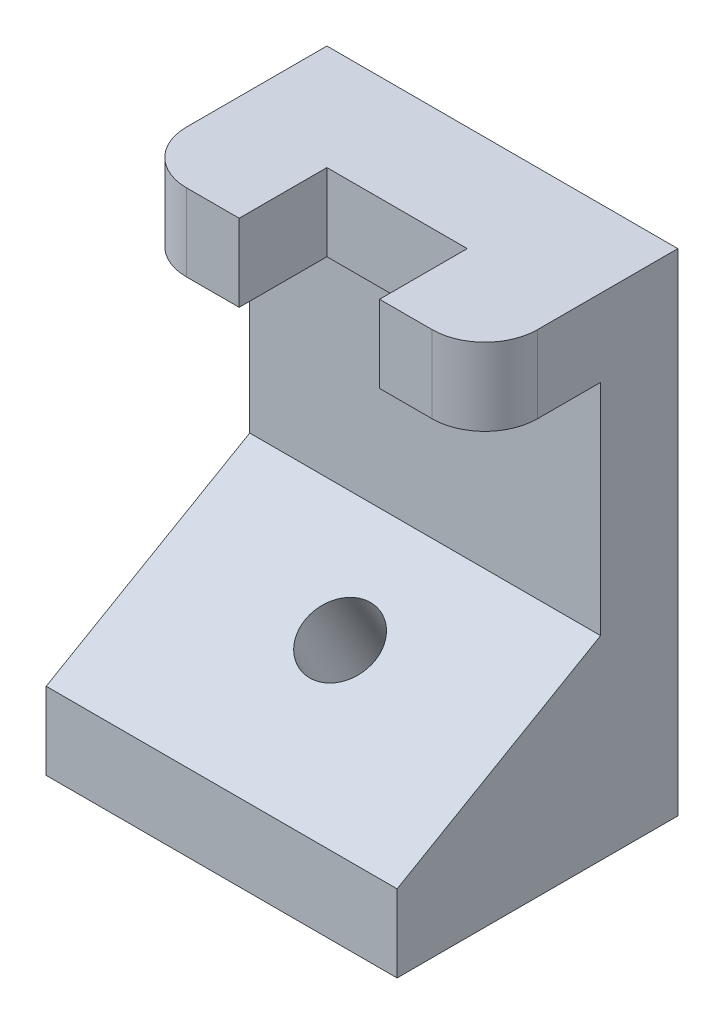
ISO-10303-21;
HEADER;
FILE_DESCRIPTION(('STEP AP214'),'2;1');
FILE_NAME('part.step','',(''),(''),'','','');
FILE_SCHEMA(('AUTOMOTIVE_DESIGN { 1 0 10303 214 1 1 1 1 }'));
ENDSEC;
DATA;
#1=APPLICATION_CONTEXT('core data for automotive mechanical design processes');
#2=APPLICATION_PROTOCOL_DEFINITION('international standard','automotive_design',2000,#1);
#3=PRODUCT_CONTEXT('',#1,'mechanical');
#4=PRODUCT('Part','Part','',(#3));
#5=PRODUCT_RELATED_PRODUCT_CATEGORY('part','',(#4));
#6=PRODUCT_DEFINITION_FORMATION('','',#4);
#7=PRODUCT_DEFINITION_CONTEXT('part definition',#1,'design');
#8=PRODUCT_DEFINITION('design','',#6,#7);
#9=PRODUCT_DEFINITION_SHAPE('','',#8);
#10=(LENGTH_UNIT() NAMED_UNIT(*) SI_UNIT(.MILLI.,.METRE.));
#11=(NAMED_UNIT(*) PLANE_ANGLE_UNIT() SI_UNIT($,.RADIAN.));
#12=(NAMED_UNIT(*) SI_UNIT($,.STERADIAN.) SOLID_ANGLE_UNIT());
#13=UNCERTAINTY_MEASURE_WITH_UNIT(LENGTH_MEASURE(1.E-05),#10,'distance_accuracy_value','');
#14=(GEOMETRIC_REPRESENTATION_CONTEXT(3) GLOBAL_UNCERTAINTY_ASSIGNED_CONTEXT((#13)) GLOBAL_UNIT_ASSIGNED_CONTEXT((#10,
#11,#12)) REPRESENTATION_CONTEXT('',''));
#15=CARTESIAN_POINT('',(0.,0.,0.));
#16=DIRECTION('',(0.,0.,1.));
#17=DIRECTION('',(1.,0.,0.));
#18=AXIS2_PLACEMENT_3D('',#15,#16,#17);
#19=CARTESIAN_POINT('',(1.,2.8,-0.500000000000001));
#20=DIRECTION('',(0.,0.,-1.));
#21=DIRECTION('',(-1.,0.,0.));
#22=AXIS2_PLACEMENT_3D('',#19,#20,#21);
#23=PLANE('',#22);
#24=DIRECTION('',(-1.,0.,0.));
#25=VECTOR('',#24,1.);
#26=CARTESIAN_POINT('',(1.,2.36,-0.500000000000001));
#27=LINE('',#26,#25);
#28=CARTESIAN_POINT('',(0.7,2.36,-0.500000000000001));
#29=VERTEX_POINT('',#28);
#30=CARTESIAN_POINT('',(0.4,2.36,-0.500000000000001));
#31=VERTEX_POINT('',#30);
#32=EDGE_CURVE('E222',#29,#31,#27,.T.);
#33=ORIENTED_EDGE('',*,*,#32,.F.);
#34=DIRECTION('',(0.,-1.,0.));
#35=VECTOR('',#34,1.);
#36=CARTESIAN_POINT('',(0.7,2.8,-0.500000000000001));
#37=LINE('',#36,#35);
#38=CARTESIAN_POINT('',(0.7,2.8,-0.500000000000001));
#39=VERTEX_POINT('',#38);
#40=EDGE_CURVE('E246',#29,#39,#37,.F.);
#41=ORIENTED_EDGE('',*,*,#40,.T.);
#42=DIRECTION('',(-1.,0.,0.));
#43=VECTOR('',#42,1.);
#44=CARTESIAN_POINT('',(1.,2.8,-0.500000000000001));
#45=LINE('',#44,#43);
#46=CARTESIAN_POINT('',(0.4,2.8,-0.500000000000001));
#47=VERTEX_POINT('',#46);
#48=EDGE_CURVE('E221',#39,#47,#45,.T.);
#49=ORIENTED_EDGE('',*,*,#48,.T.);
#50=DIRECTION('',(0.,1.,0.));
#51=VECTOR('',#50,1.);
#52=CARTESIAN_POINT('',(0.4,1.8,-0.500000000000001));
#53=LINE('',#52,#51);
#54=EDGE_CURVE('E163',#31,#47,#53,.T.);
#55=ORIENTED_EDGE('',*,*,#54,.F.);
#56=EDGE_LOOP('',(#33,#41,#49,#55));
#57=FACE_BOUND('',#56,.T.);
#58=ADVANCED_FACE('F44',(#57),#23,.F.);
#59=CARTESIAN_POINT('',(1.,0.,0.));
#60=DIRECTION('',(0.,0.,-1.));
#61=DIRECTION('',(-1.,0.,0.));
#62=AXIS2_PLACEMENT_3D('',#59,#60,#61);
#63=PLANE('',#62);
#64=DIRECTION('',(0.,-1.,0.));
#65=VECTOR('',#64,1.);
#66=CARTESIAN_POINT('',(-1.,0.,0.));
#67=LINE('',#66,#65);
#68=CARTESIAN_POINT('',(-1.,0.44,0.));
#69=VERTEX_POINT('',#68);
#70=CARTESIAN_POINT('',(-1.,0.,0.));
#71=VERTEX_POINT('',#70);
#72=EDGE_CURVE('E176',#69,#71,#67,.T.);
#73=ORIENTED_EDGE('',*,*,#72,.T.);
#74=DIRECTION('',(-1.,0.,0.));
#75=VECTOR('',#74,1.);
#76=CARTESIAN_POINT('',(1.,0.,0.));
#77=LINE('',#76,#75);
#78=CARTESIAN_POINT('',(1.,0.,0.));
#79=VERTEX_POINT('',#78);
#80=EDGE_CURVE('E235',#79,#71,#77,.T.);
#81=ORIENTED_EDGE('',*,*,#80,.F.);
#82=DIRECTION('',(0.,-1.,0.));
#83=VECTOR('',#82,1.);
#84=CARTESIAN_POINT('',(1.,0.,0.));
#85=LINE('',#84,#83);
#86=CARTESIAN_POINT('',(1.,0.44,0.));
#87=VERTEX_POINT('',#86);
#88=EDGE_CURVE('E182',#87,#79,#85,.T.);
#89=ORIENTED_EDGE('',*,*,#88,.F.);
#90=DIRECTION('',(-1.,0.,0.));
#91=VECTOR('',#90,1.);
#92=CARTESIAN_POINT('',(1.,0.44,0.));
#93=LINE('',#92,#91);
#94=EDGE_CURVE('E196',#87,#69,#93,.T.);
#95=ORIENTED_EDGE('',*,*,#94,.T.);
#96=EDGE_LOOP('',(#73,#81,#89,#95));
#97=FACE_BOUND('',#96,.T.);
#98=ADVANCED_FACE('F274',(#97),#63,.F.);
#99=CARTESIAN_POINT('',(1.,0.,0.));
#100=DIRECTION('',(0.,1.,0.));
#101=DIRECTION('',(0.,0.,1.));
#102=AXIS2_PLACEMENT_3D('',#99,#100,#101);
#103=PLANE('',#102);
#104=CARTESIAN_POINT('',(0.,0.,-1.15406848361773));
#105=DIRECTION('',(0.,1.,0.));
#106=DIRECTION('',(0.,0.,1.));
#107=AXIS2_PLACEMENT_3D('',#104,#105,#106);
#108=ELLIPSE('',#107,0.230940107675851,0.2);
#109=CARTESIAN_POINT('',(0.,0.,-0.923128375941875));
#110=VERTEX_POINT('',#109);
#111=EDGE_CURVE('E170',#110,#110,#108,.T.);
#112=ORIENTED_EDGE('',*,*,#111,.T.);
#113=EDGE_LOOP('',(#112));
#114=FACE_BOUND('',#113,.T.);
#115=DIRECTION('',(0.,0.,-1.));
#116=VECTOR('',#115,1.);
#117=CARTESIAN_POINT('',(-1.,0.,0.));
#118=LINE('',#117,#116);
#119=CARTESIAN_POINT('',(-1.,0.,-1.6));
#120=VERTEX_POINT('',#119);
#121=EDGE_CURVE('E203',#71,#120,#118,.T.);
#122=ORIENTED_EDGE('',*,*,#121,.T.);
#123=DIRECTION('',(-1.,0.,0.));
#124=VECTOR('',#123,1.);
#125=CARTESIAN_POINT('',(1.,0.,-1.6));
#126=LINE('',#125,#124);
#127=CARTESIAN_POINT('',(1.,0.,-1.6));
#128=VERTEX_POINT('',#127);
#129=EDGE_CURVE('E226',#128,#120,#126,.T.);
#130=ORIENTED_EDGE('',*,*,#129,.F.);
#131=DIRECTION('',(0.,0.,-1.));
#132=VECTOR('',#131,1.);
#133=CARTESIAN_POINT('',(1.,0.,0.));
#134=LINE('',#133,#132);
#135=EDGE_CURVE('E184',#79,#128,#134,.T.);
#136=ORIENTED_EDGE('',*,*,#135,.F.);
#137=ORIENTED_EDGE('',*,*,#80,.T.);
#138=EDGE_LOOP('',(#122,#130,#136,#137));
#139=FACE_BOUND('',#138,.T.);
#140=ADVANCED_FACE('F282',(#114,#139),#103,.F.);
#141=CARTESIAN_POINT('',(1.,0.,-1.6));
#142=DIRECTION('',(0.,0.,1.));
#143=DIRECTION('',(1.,0.,0.));
#144=AXIS2_PLACEMENT_3D('',#141,#142,#143);
#145=PLANE('',#144);
#146=DIRECTION('',(0.,1.,0.));
#147=VECTOR('',#146,1.);
#148=CARTESIAN_POINT('',(-1.,0.,-1.6));
#149=LINE('',#148,#147);
#150=CARTESIAN_POINT('',(-1.,2.8,-1.6));
#151=VERTEX_POINT('',#150);
#152=EDGE_CURVE('E201',#120,#151,#149,.T.);
#153=ORIENTED_EDGE('',*,*,#152,.T.);
#154=DIRECTION('',(-1.,0.,0.));
#155=VECTOR('',#154,1.);
#156=CARTESIAN_POINT('',(1.,2.8,-1.6));
#157=LINE('',#156,#155);
#158=CARTESIAN_POINT('',(1.,2.8,-1.6));
#159=VERTEX_POINT('',#158);
#160=EDGE_CURVE('E227',#159,#151,#157,.T.);
#161=ORIENTED_EDGE('',*,*,#160,.F.);
#162=DIRECTION('',(0.,1.,0.));
#163=VECTOR('',#162,1.);
#164=CARTESIAN_POINT('',(1.,0.,-1.6));
#165=LINE('',#164,#163);
#166=EDGE_CURVE('E189',#128,#159,#165,.T.);
#167=ORIENTED_EDGE('',*,*,#166,.F.);
#168=ORIENTED_EDGE('',*,*,#129,.T.);
#169=EDGE_LOOP('',(#153,#161,#167,#168));
#170=FACE_BOUND('',#169,.T.);
#171=ADVANCED_FACE('F294',(#170),#145,.F.);
#172=CARTESIAN_POINT('',(1.,2.8,-1.6));
#173=DIRECTION('',(0.,-1.,0.));
#174=DIRECTION('',(0.,0.,-1.));
#175=AXIS2_PLACEMENT_3D('',#172,#173,#174);
#176=PLANE('',#175);
#177=DIRECTION('',(0.,0.,1.));
#178=VECTOR('',#177,1.);
#179=CARTESIAN_POINT('',(-1.,2.8,-1.6));
#180=LINE('',#179,#178);
#181=CARTESIAN_POINT('',(-1.,2.8,-0.800000000000001));
#182=VERTEX_POINT('',#181);
#183=EDGE_CURVE('E202',#151,#182,#180,.T.);
#184=ORIENTED_EDGE('',*,*,#183,.T.);
#185=CARTESIAN_POINT('',(-0.7,2.8,-0.800000000000001));
#186=DIRECTION('',(0.,-1.,0.));
#187=DIRECTION('',(0.,0.,-1.));
#188=AXIS2_PLACEMENT_3D('',#185,#186,#187);
#189=CIRCLE('',#188,0.3);
#190=CARTESIAN_POINT('',(-0.7,2.8,-0.500000000000001));
#191=VERTEX_POINT('',#190);
#192=EDGE_CURVE('E11',#182,#191,#189,.F.);
#193=ORIENTED_EDGE('',*,*,#192,.T.);
#194=CARTESIAN_POINT('',(-0.4,2.8,-0.500000000000001));
#195=VERTEX_POINT('',#194);
#196=EDGE_CURVE('E224',#195,#191,#45,.T.);
#197=ORIENTED_EDGE('',*,*,#196,.F.);
#198=DIRECTION('',(0.,0.,1.));
#199=VECTOR('',#198,1.);
#200=CARTESIAN_POINT('',(-0.4,2.8,-1.));
#201=LINE('',#200,#199);
#202=CARTESIAN_POINT('',(-0.4,2.8,-1.));
#203=VERTEX_POINT('',#202);
#204=EDGE_CURVE('E160',#203,#195,#201,.T.);
#205=ORIENTED_EDGE('',*,*,#204,.F.);
#206=DIRECTION('',(-1.,0.,0.));
#207=VECTOR('',#206,1.);
#208=CARTESIAN_POINT('',(0.4,2.8,-1.));
#209=LINE('',#208,#207);
#210=CARTESIAN_POINT('',(0.4,2.8,-1.));
#211=VERTEX_POINT('',#210);
#212=EDGE_CURVE('E149',#211,#203,#209,.T.);
#213=ORIENTED_EDGE('',*,*,#212,.F.);
#214=DIRECTION('',(0.,0.,-1.));
#215=VECTOR('',#214,1.);
#216=CARTESIAN_POINT('',(0.4,2.8,-1.));
#217=LINE('',#216,#215);
#218=EDGE_CURVE('E161',#47,#211,#217,.T.);
#219=ORIENTED_EDGE('',*,*,#218,.F.);
#220=ORIENTED_EDGE('',*,*,#48,.F.);
#221=CARTESIAN_POINT('',(0.7,2.8,-0.800000000000001));
#222=DIRECTION('',(0.,-1.,0.));
#223=DIRECTION('',(0.,0.,-1.));
#224=AXIS2_PLACEMENT_3D('',#221,#222,#223);
#225=CIRCLE('',#224,0.3);
#226=CARTESIAN_POINT('',(1.,2.8,-0.800000000000001));
#227=VERTEX_POINT('',#226);
#228=EDGE_CURVE('E247',#39,#227,#225,.F.);
#229=ORIENTED_EDGE('',*,*,#228,.T.);
#230=DIRECTION('',(0.,0.,1.));
#231=VECTOR('',#230,1.);
#232=CARTESIAN_POINT('',(1.,2.8,-1.6));
#233=LINE('',#232,#231);
#234=EDGE_CURVE('E186',#159,#227,#233,.T.);
#235=ORIENTED_EDGE('',*,*,#234,.F.);
#236=ORIENTED_EDGE('',*,*,#160,.T.);
#237=EDGE_LOOP('',(#184,#193,#197,#205,#213,#219,#220,#229,#235,#236));
#238=FACE_BOUND('',#237,.T.);
#239=ADVANCED_FACE('F166',(#238),#176,.F.);
#240=ORIENTED_EDGE('',*,*,#196,.T.);
#241=DIRECTION('',(0.,-1.,0.));
#242=VECTOR('',#241,1.);
#243=CARTESIAN_POINT('',(-0.7,2.36,-0.500000000000001));
#244=LINE('',#243,#242);
#245=CARTESIAN_POINT('',(-0.7,2.36,-0.500000000000001));
#246=VERTEX_POINT('',#245);
#247=EDGE_CURVE('E249',#191,#246,#244,.T.);
#248=ORIENTED_EDGE('',*,*,#247,.T.);
#249=CARTESIAN_POINT('',(-0.4,2.36,-0.500000000000001));
#250=VERTEX_POINT('',#249);
#251=EDGE_CURVE('E219',#250,#246,#27,.T.);
#252=ORIENTED_EDGE('',*,*,#251,.F.);
#253=DIRECTION('',(0.,1.,0.));
#254=VECTOR('',#253,1.);
#255=CARTESIAN_POINT('',(-0.4,1.8,-0.500000000000001));
#256=LINE('',#255,#254);
#257=EDGE_CURVE('E180',#250,#195,#256,.T.);
#258=ORIENTED_EDGE('',*,*,#257,.T.);
#259=EDGE_LOOP('',(#240,#248,#252,#258));
#260=FACE_BOUND('',#259,.T.);
#261=ADVANCED_FACE('F260',(#260),#23,.F.);
#262=CARTESIAN_POINT('',(1.,2.36,-0.500000000000001));
#263=DIRECTION('',(0.,1.,0.));
#264=DIRECTION('',(0.,0.,1.));
#265=AXIS2_PLACEMENT_3D('',#262,#263,#264);
#266=PLANE('',#265);
#267=ORIENTED_EDGE('',*,*,#251,.T.);
#268=CARTESIAN_POINT('',(-0.7,2.36,-0.800000000000001));
#269=DIRECTION('',(0.,1.,0.));
#270=DIRECTION('',(0.,0.,1.));
#271=AXIS2_PLACEMENT_3D('',#268,#269,#270);
#272=CIRCLE('',#271,0.3);
#273=CARTESIAN_POINT('',(-1.,2.36,-0.8));
#274=VERTEX_POINT('',#273);
#275=EDGE_CURVE('E70',#246,#274,#272,.F.);
#276=ORIENTED_EDGE('',*,*,#275,.T.);
#277=DIRECTION('',(0.,0.,-1.));
#278=VECTOR('',#277,1.);
#279=CARTESIAN_POINT('',(-1.,2.36,-0.500000000000001));
#280=LINE('',#279,#278);
#281=CARTESIAN_POINT('',(-1.,2.36,-1.16));
#282=VERTEX_POINT('',#281);
#283=EDGE_CURVE('E210',#274,#282,#280,.T.);
#284=ORIENTED_EDGE('',*,*,#283,.T.);
#285=DIRECTION('',(-1.,0.,0.));
#286=VECTOR('',#285,1.);
#287=CARTESIAN_POINT('',(1.,2.36,-1.16));
#288=LINE('',#287,#286);
#289=CARTESIAN_POINT('',(1.,2.36,-1.16));
#290=VERTEX_POINT('',#289);
#291=EDGE_CURVE('E220',#290,#282,#288,.T.);
#292=ORIENTED_EDGE('',*,*,#291,.F.);
#293=DIRECTION('',(0.,0.,-1.));
#294=VECTOR('',#293,1.);
#295=CARTESIAN_POINT('',(1.,2.36,-0.500000000000001));
#296=LINE('',#295,#294);
#297=CARTESIAN_POINT('',(1.,2.36,-0.8));
#298=VERTEX_POINT('',#297);
#299=EDGE_CURVE('E195',#298,#290,#296,.T.);
#300=ORIENTED_EDGE('',*,*,#299,.F.);
#301=CARTESIAN_POINT('',(0.7,2.36,-0.800000000000001));
#302=DIRECTION('',(0.,1.,0.));
#303=DIRECTION('',(0.,0.,1.));
#304=AXIS2_PLACEMENT_3D('',#301,#302,#303);
#305=CIRCLE('',#304,0.3);
#306=EDGE_CURVE('E241',#298,#29,#305,.F.);
#307=ORIENTED_EDGE('',*,*,#306,.T.);
#308=ORIENTED_EDGE('',*,*,#32,.T.);
#309=DIRECTION('',(0.,0.,-1.));
#310=VECTOR('',#309,1.);
#311=CARTESIAN_POINT('',(0.4,2.36,-0.500000000000001));
#312=LINE('',#311,#310);
#313=CARTESIAN_POINT('',(0.4,2.36,-1.));
#314=VERTEX_POINT('',#313);
#315=EDGE_CURVE('E239',#31,#314,#312,.T.);
#316=ORIENTED_EDGE('',*,*,#315,.T.);
#317=DIRECTION('',(-1.,0.,0.));
#318=VECTOR('',#317,1.);
#319=CARTESIAN_POINT('',(1.,2.36,-1.));
#320=LINE('',#319,#318);
#321=CARTESIAN_POINT('',(-0.4,2.36,-1.));
#322=VERTEX_POINT('',#321);
#323=EDGE_CURVE('E155',#314,#322,#320,.T.);
#324=ORIENTED_EDGE('',*,*,#323,.T.);
#325=DIRECTION('',(0.,0.,1.));
#326=VECTOR('',#325,1.);
#327=CARTESIAN_POINT('',(-0.4,2.36,-0.500000000000001));
#328=LINE('',#327,#326);
#329=EDGE_CURVE('E237',#322,#250,#328,.T.);
#330=ORIENTED_EDGE('',*,*,#329,.T.);
#331=EDGE_LOOP('',(#267,#276,#284,#292,#300,#307,#308,#316,#324,#330));
#332=FACE_BOUND('',#331,.T.);
#333=ADVANCED_FACE('F257',(#332),#266,.F.);
#334=CARTESIAN_POINT('',(1.,2.36,-1.16));
#335=DIRECTION('',(0.,0.,-1.));
#336=DIRECTION('',(0.,1.,0.));
#337=AXIS2_PLACEMENT_3D('',#334,#335,#336);
#338=PLANE('',#337);
#339=DIRECTION('',(0.,-1.,0.));
#340=VECTOR('',#339,1.);
#341=CARTESIAN_POINT('',(-1.,2.36,-1.16));
#342=LINE('',#341,#340);
#343=CARTESIAN_POINT('',(-1.,1.10972631225997,-1.16));
#344=VERTEX_POINT('',#343);
#345=EDGE_CURVE('E207',#282,#344,#342,.T.);
#346=ORIENTED_EDGE('',*,*,#345,.T.);
#347=DIRECTION('',(-1.,0.,0.));
#348=VECTOR('',#347,1.);
#349=CARTESIAN_POINT('',(1.,1.10972631225997,-1.16));
#350=LINE('',#349,#348);
#351=CARTESIAN_POINT('',(1.,1.10972631225997,-1.16));
#352=VERTEX_POINT('',#351);
#353=EDGE_CURVE('E212',#352,#344,#350,.T.);
#354=ORIENTED_EDGE('',*,*,#353,.F.);
#355=DIRECTION('',(0.,-1.,0.));
#356=VECTOR('',#355,1.);
#357=CARTESIAN_POINT('',(1.,2.36,-1.16));
#358=LINE('',#357,#356);
#359=EDGE_CURVE('E193',#290,#352,#358,.T.);
#360=ORIENTED_EDGE('',*,*,#359,.F.);
#361=ORIENTED_EDGE('',*,*,#291,.T.);
#362=EDGE_LOOP('',(#346,#354,#360,#361));
#363=FACE_BOUND('',#362,.T.);
#364=ADVANCED_FACE('F291',(#363),#338,.F.);
#365=CARTESIAN_POINT('',(1.,0.44,0.));
#366=DIRECTION('',(0.,-0.866025403784438,-0.500000000000001));
#367=DIRECTION('',(0.,0.500000000000001,-0.866025403784438));
#368=AXIS2_PLACEMENT_3D('',#365,#366,#367);
#369=PLANE('',#368);
#370=CARTESIAN_POINT('',(0.,0.829726312259968,-0.675025773880716));
#371=DIRECTION('',(0.,0.866025403784438,0.500000000000001));
#372=DIRECTION('',(0.,-0.500000000000001,0.866025403784438));
#373=AXIS2_PLACEMENT_3D('',#370,#371,#372);
#374=CIRCLE('',#373,0.2);
#375=CARTESIAN_POINT('',(0.,0.729726312259968,-0.501820693123828));
#376=VERTEX_POINT('',#375);
#377=EDGE_CURVE('E540',#376,#376,#374,.T.);
#378=ORIENTED_EDGE('',*,*,#377,.F.);
#379=EDGE_LOOP('',(#378));
#380=FACE_BOUND('',#379,.T.);
#381=DIRECTION('',(0.,-0.500000000000001,0.866025403784438));
#382=VECTOR('',#381,1.);
#383=CARTESIAN_POINT('',(-1.,0.44,0.));
#384=LINE('',#383,#382);
#385=EDGE_CURVE('E183',#344,#69,#384,.T.);
#386=ORIENTED_EDGE('',*,*,#385,.T.);
#387=ORIENTED_EDGE('',*,*,#94,.F.);
#388=DIRECTION('',(0.,-0.500000000000001,0.866025403784438));
#389=VECTOR('',#388,1.);
#390=CARTESIAN_POINT('',(1.,0.44,0.));
#391=LINE('',#390,#389);
#392=EDGE_CURVE('E198',#352,#87,#391,.T.);
#393=ORIENTED_EDGE('',*,*,#392,.F.);
#394=ORIENTED_EDGE('',*,*,#353,.T.);
#395=EDGE_LOOP('',(#386,#387,#393,#394));
#396=FACE_BOUND('',#395,.T.);
#397=ADVANCED_FACE('F322',(#380,#396),#369,.F.);
#398=CARTESIAN_POINT('',(1.,0.,0.));
#399=DIRECTION('',(-1.,0.,0.));
#400=DIRECTION('',(0.,0.,1.));
#401=AXIS2_PLACEMENT_3D('',#398,#399,#400);
#402=PLANE('',#401);
#403=ORIENTED_EDGE('',*,*,#234,.T.);
#404=DIRECTION('',(0.,-1.,0.));
#405=VECTOR('',#404,1.);
#406=CARTESIAN_POINT('',(1.,0.,-0.800000000000001));
#407=LINE('',#406,#405);
#408=EDGE_CURVE('E242',#227,#298,#407,.T.);
#409=ORIENTED_EDGE('',*,*,#408,.T.);
#410=ORIENTED_EDGE('',*,*,#299,.T.);
#411=ORIENTED_EDGE('',*,*,#359,.T.);
#412=ORIENTED_EDGE('',*,*,#392,.T.);
#413=ORIENTED_EDGE('',*,*,#88,.T.);
#414=ORIENTED_EDGE('',*,*,#135,.T.);
#415=ORIENTED_EDGE('',*,*,#166,.T.);
#416=EDGE_LOOP('',(#403,#409,#410,#411,#412,#413,#414,#415));
#417=FACE_BOUND('',#416,.T.);
#418=ADVANCED_FACE('F320',(#417),#402,.F.);
#419=CARTESIAN_POINT('',(-1.,0.,0.));
#420=DIRECTION('',(-1.,0.,0.));
#421=DIRECTION('',(0.,0.,1.));
#422=AXIS2_PLACEMENT_3D('',#419,#420,#421);
#423=PLANE('',#422);
#424=ORIENTED_EDGE('',*,*,#283,.F.);
#425=DIRECTION('',(0.,-1.,0.));
#426=VECTOR('',#425,1.);
#427=CARTESIAN_POINT('',(-1.,2.8,-0.800000000000001));
#428=LINE('',#427,#426);
#429=EDGE_CURVE('E52',#274,#182,#428,.F.);
#430=ORIENTED_EDGE('',*,*,#429,.T.);
#431=ORIENTED_EDGE('',*,*,#183,.F.);
#432=ORIENTED_EDGE('',*,*,#152,.F.);
#433=ORIENTED_EDGE('',*,*,#121,.F.);
#434=ORIENTED_EDGE('',*,*,#72,.F.);
#435=ORIENTED_EDGE('',*,*,#385,.F.);
#436=ORIENTED_EDGE('',*,*,#345,.F.);
#437=EDGE_LOOP('',(#424,#430,#431,#432,#433,#434,#435,#436));
#438=FACE_BOUND('',#437,.T.);
#439=ADVANCED_FACE('F314',(#438),#423,.T.);
#440=CARTESIAN_POINT('',(0.4,1.8,-1.));
#441=DIRECTION('',(1.,0.,0.));
#442=DIRECTION('',(0.,0.,-1.));
#443=AXIS2_PLACEMENT_3D('',#440,#441,#442);
#444=PLANE('',#443);
#445=ORIENTED_EDGE('',*,*,#54,.T.);
#446=ORIENTED_EDGE('',*,*,#218,.T.);
#447=DIRECTION('',(0.,1.,0.));
#448=VECTOR('',#447,1.);
#449=CARTESIAN_POINT('',(0.4,1.8,-1.));
#450=LINE('',#449,#448);
#451=EDGE_CURVE('E144',#314,#211,#450,.T.);
#452=ORIENTED_EDGE('',*,*,#451,.F.);
#453=ORIENTED_EDGE('',*,*,#315,.F.);
#454=EDGE_LOOP('',(#445,#446,#452,#453));
#455=FACE_BOUND('',#454,.T.);
#456=ADVANCED_FACE('F165',(#455),#444,.F.);
#457=CARTESIAN_POINT('',(-0.4,1.8,-1.));
#458=DIRECTION('',(-1.,0.,0.));
#459=DIRECTION('',(0.,0.,1.));
#460=AXIS2_PLACEMENT_3D('',#457,#458,#459);
#461=PLANE('',#460);
#462=DIRECTION('',(0.,1.,0.));
#463=VECTOR('',#462,1.);
#464=CARTESIAN_POINT('',(-0.4,1.8,-1.));
#465=LINE('',#464,#463);
#466=EDGE_CURVE('E156',#322,#203,#465,.T.);
#467=ORIENTED_EDGE('',*,*,#466,.T.);
#468=ORIENTED_EDGE('',*,*,#204,.T.);
#469=ORIENTED_EDGE('',*,*,#257,.F.);
#470=ORIENTED_EDGE('',*,*,#329,.F.);
#471=EDGE_LOOP('',(#467,#468,#469,#470));
#472=FACE_BOUND('',#471,.T.);
#473=ADVANCED_FACE('F263',(#472),#461,.F.);
#474=CARTESIAN_POINT('',(0.4,1.8,-1.));
#475=DIRECTION('',(0.,0.,-1.));
#476=DIRECTION('',(-1.,0.,0.));
#477=AXIS2_PLACEMENT_3D('',#474,#475,#476);
#478=PLANE('',#477);
#479=ORIENTED_EDGE('',*,*,#451,.T.);
#480=ORIENTED_EDGE('',*,*,#212,.T.);
#481=ORIENTED_EDGE('',*,*,#466,.F.);
#482=ORIENTED_EDGE('',*,*,#323,.F.);
#483=EDGE_LOOP('',(#479,#480,#481,#482));
#484=FACE_BOUND('',#483,.T.);
#485=ADVANCED_FACE('F150',(#484),#478,.F.);
#486=CARTESIAN_POINT('',(0.7,0.,-0.800000000000001));
#487=DIRECTION('',(0.,-1.,0.));
#488=DIRECTION('',(0.,0.,-1.));
#489=AXIS2_PLACEMENT_3D('',#486,#487,#488);
#490=CYLINDRICAL_SURFACE('',#489,0.3);
#491=ORIENTED_EDGE('',*,*,#228,.F.);
#492=ORIENTED_EDGE('',*,*,#40,.F.);
#493=ORIENTED_EDGE('',*,*,#306,.F.);
#494=ORIENTED_EDGE('',*,*,#408,.F.);
#495=EDGE_LOOP('',(#491,#492,#493,#494));
#496=FACE_BOUND('',#495,.T.);
#497=ADVANCED_FACE('F266',(#496),#490,.T.);
#498=CARTESIAN_POINT('',(-0.7,2.8,-0.800000000000001));
#499=DIRECTION('',(0.,1.,0.));
#500=DIRECTION('',(0.,0.,1.));
#501=AXIS2_PLACEMENT_3D('',#498,#499,#500);
#502=CYLINDRICAL_SURFACE('',#501,0.3);
#503=ORIENTED_EDGE('',*,*,#192,.F.);
#504=ORIENTED_EDGE('',*,*,#429,.F.);
#505=ORIENTED_EDGE('',*,*,#275,.F.);
#506=ORIENTED_EDGE('',*,*,#247,.F.);
#507=EDGE_LOOP('',(#503,#504,#505,#506));
#508=FACE_BOUND('',#507,.T.);
#509=ADVANCED_FACE('F50',(#508),#502,.T.);
#510=CARTESIAN_POINT('',(0.,-0.902324495308908,-1.67502577388072));
#511=DIRECTION('',(0.,0.866025403784438,0.500000000000001));
#512=DIRECTION('',(0.,-0.500000000000001,0.866025403784438));
#513=AXIS2_PLACEMENT_3D('',#510,#511,#512);
#514=CYLINDRICAL_SURFACE('',#513,0.2);
#515=ORIENTED_EDGE('',*,*,#377,.T.);
#516=EDGE_LOOP('',(#515));
#517=FACE_BOUND('',#516,.T.);
#518=ORIENTED_EDGE('',*,*,#111,.F.);
#519=EDGE_LOOP('',(#518));
#520=FACE_BOUND('',#519,.T.);
#521=ADVANCED_FACE('F264',(#517,#520),#514,.F.);
#522=CLOSED_SHELL('',(#58,#98,#140,#171,#239,#261,#333,#364,#397,#418,#439,#456,#473,#485,#497,
#509,#521));
#523=MANIFOLD_SOLID_BREP('B2',#522);
#524=ADVANCED_BREP_SHAPE_REPRESENTATION('',(#18,#523),#14);
#525=SHAPE_DEFINITION_REPRESENTATION(#9,#524);
ENDSEC;
END-ISO-10303-21;
